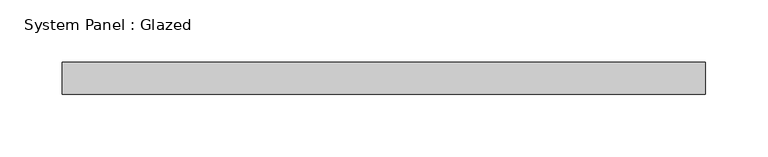
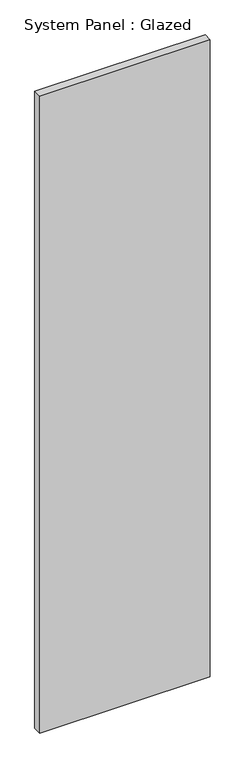
"""IFC4 building model written with IfcOpenShell, lengths in millimetres: plate geometry, System Panel : Glazed."""

from ifc_helpers import new_model, si_unit, origin, origin_with_axes, place, context, project, spatial, polyline, outline, extrude, source, transform, mapped, element, save


def system_panel_glazed_f1c144f9(model_context):
    return source(origin(), model_context, "Body", "SweptSolid", [
        extrude(outline(polyline([(257.6030168, 19.05), (-257.6030168, 19.05), (-257.6030168, 44.45), (257.6030168, 44.45), (257.6030168, 19.05)])), origin_with_axes(), (0.0, 0.0, 1.0), 2032.0),
    ])


if __name__ == "__main__":
    model = new_model("IFC4")
    model_context = context("Model", 3, world=origin())
    ifc_project = project(units=[si_unit("LENGTHUNIT", "METRE", prefix="MILLI")], contexts=[model_context])
    site = spatial("IfcSite", under=ifc_project)
    building = spatial("IfcBuilding", under=site)
    placement = place(None, origin())
    system_panel_glazed_shape = system_panel_glazed_f1c144f9(model_context)
    element("IfcPlate", 1, ObjectType="System Panel : Glazed", at=placement, inside=building, context=model_context, shape_type="MappedRepresentation", body=[
        mapped(system_panel_glazed_shape, transform((0.0, 0.0, 0.0), x_axis=(1.0, 0.0, 0.0), y_axis=(0.0, 1.0, 0.0), z_axis=(0.0, 0.0, 1.0))),
    ])
    save(model, "model.ifc")

# Revit data of these elements
# Type "System Panel : Glazed"
#   Construction Type Id = "GSP4R"
#   Analytic Construction = "1/8 in Pilkington single glazing"
#   Visual Light Transmittance = 0.9
#   Solar Heat Gain Coefficient = 0.86
#   Heat Transfer Coefficient (U) = 1.18115 BTU/(h·ft²·°F)
# Element 1 (IfcPlate, "System Panel : Glazed")
#   Materials on its faces: "Glass"
# Materials
#   "Glass": class "Glass", colour RGB 0 128 192, transparency 0.75, Description = "Soda Lime Glass", Cost = 0
